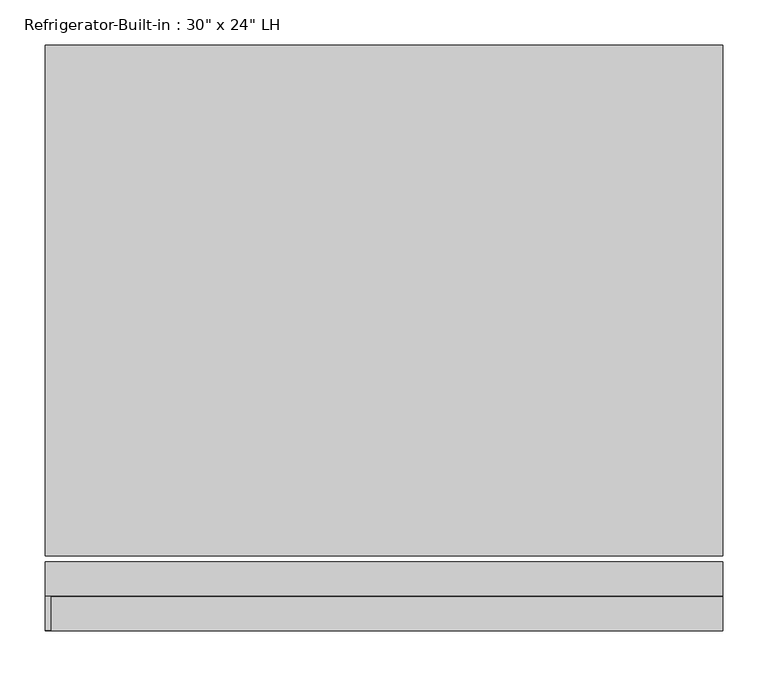
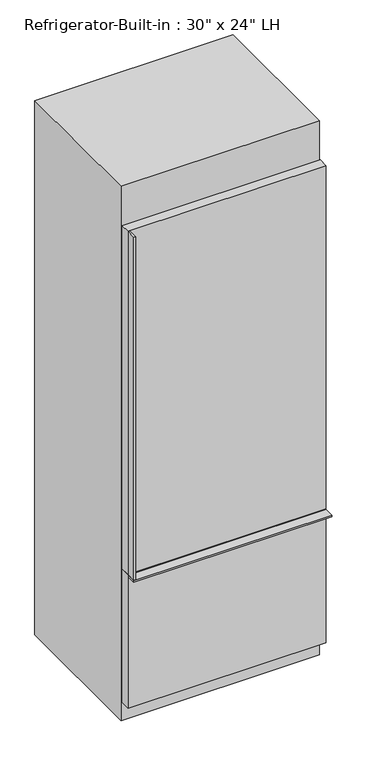
"""IFC4 building model written with IfcOpenShell, lengths in millimetres: proxy geometry."""

from ifc_helpers import new_model, si_unit, frame, origin, origin_with_axes, place, context, project, spatial, polyline, outline, extrude, source, transform, mapped, element, save


def proxy_19935bb1(model_context):
    return source(origin(), model_context, "Body", "SweptSolid", [
        extrude(outline(polyline([(374.65, 290.1239715), (374.65, -275.0260285), (-374.65, -275.0260285), (-374.65, 290.1239715), (374.65, 290.1239715)])), origin_with_axes(), (0.0, 0.0, 1.0), 2133.6),
        extrude(outline(polyline([(374.65, -281.3760285), (374.65, -319.4760285), (-374.65, -319.4760285), (-374.65, -281.3760285), (374.65, -281.3760285)])), frame((0.0, 0.0, 611.1875), z_axis=(0.0, 0.0, 1.0), x_axis=(1.0, 0.0, 0.0)), (0.0, 0.0, 1.0), 1370.0125),
        extrude(outline(polyline([(374.65, -281.3760285), (374.65, -319.4760285), (-374.65, -319.4760285), (-374.65, -281.3760285), (374.65, -281.3760285)])), frame((0.0, 0.0, 76.2), z_axis=(0.0, 0.0, 1.0), x_axis=(1.0, 0.0, 0.0)), (0.0, 0.0, 1.0), 531.8125),
        extrude(outline(polyline([(374.65, -319.4760285), (374.65, -357.5760285), (-374.65, -357.5760285), (-374.65, -319.4760285), (374.65, -319.4760285)])), frame((0.0, 0.0, 601.6625), z_axis=(0.0, 0.0, 1.0), x_axis=(1.0, 0.0, 0.0)), (0.0, 0.0, 1.0), 6.35),
        extrude(outline(polyline([(-374.65, -319.4760285), (-368.3, -319.4760285), (-368.3, -357.5760285), (-374.65, -357.5760285), (-374.65, -319.4760285)])), frame((0.0, 0.0, 611.1875), z_axis=(0.0, 0.0, 1.0), x_axis=(1.0, 0.0, 0.0)), (0.0, 0.0, 1.0), 1370.0125),
    ])


if __name__ == "__main__":
    model = new_model("IFC4")
    model_context = context("Model", 3, world=origin())
    ifc_project = project(units=[si_unit("LENGTHUNIT", "METRE", prefix="MILLI")], contexts=[model_context])
    site = spatial("IfcSite", under=ifc_project)
    building = spatial("IfcBuilding", under=site)
    placement = place(None, origin())
    proxy_shape = proxy_19935bb1(model_context)
    element("IfcBuildingElementProxy", 1, Name="Refrigerator-Built-in : 30\" x 24\" LH", ObjectType="Refrigerator-Built-in : 30\" x 24\" LH", at=placement, inside=building, context=model_context, shape_type="MappedRepresentation", body=[
        mapped(proxy_shape, transform((0.0, 0.0, 0.0), x_axis=(1.0, 0.0, 0.0), y_axis=(0.0, 1.0, 0.0), z_axis=(0.0, 0.0, 1.0))),
    ])
    save(model, "model.ifc")

# Revit data of these elements
# Type "Refrigerator-Built-in : 30\" x 24\" LH"
#   Assembly Code = "E1090400"
#   Depth = 2 ft
#   Handle = 0.020833 ft
#   Height = 7 ft
#   Top Door Height = 5 ft
#   Width = 2.458333 ft
#   Material = Metal - Paint Finish - Ivory,Glossy
#   Default Elevation = 0
# Element 1 (IfcBuildingElementProxy, "Refrigerator-Built-in : 30\" x 24\" LH")
#   Materials on its faces: "Metal - Paint Finish - Ivory,Glossy", "Metal - Chrome"
# Materials
#   "Metal - Paint Finish - Ivory,Glossy": colour RGB 247 247 239, transparency 0
#   "Metal - Chrome": class "Metal", colour RGB 247 247 247, transparency 0
